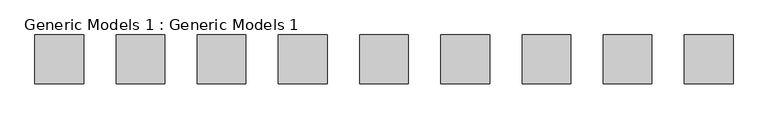
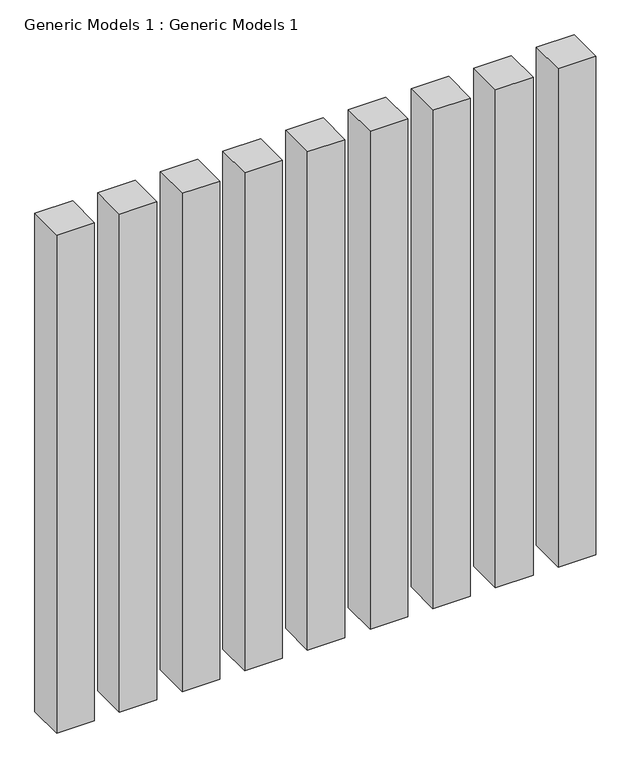
"""IFC4 building model written with IfcOpenShell, lengths in millimetres: proxy geometry, Generic Models 1 : Generic Models 1."""

from ifc_helpers import new_model, si_unit, origin, origin_with_axes, place, context, project, spatial, polyline, outline, extrude, source, transform, mapped, element, save


def generic_models_1_generic_models_1_04f99ef1(model_context):
    return source(origin(), model_context, "Body", "SweptSolid", [
        extrude(outline(polyline([(23542.6546318, -2836.165108), (23314.0546318, -2836.165108), (23314.0546318, -2607.565108), (23542.6546318, -2607.565108), (23542.6546318, -2836.165108)])), origin_with_axes(), (0.0, 0.0, 1.0), 3200.4),
        extrude(outline(polyline([(23923.6546318, -2836.165108), (23695.0546318, -2836.165108), (23695.0546318, -2607.565108), (23923.6546318, -2607.565108), (23923.6546318, -2836.165108)])), origin_with_axes(), (0.0, 0.0, 1.0), 3200.4),
        extrude(outline(polyline([(24304.6546318, -2836.165108), (24076.0546318, -2836.165108), (24076.0546318, -2607.565108), (24304.6546318, -2607.565108), (24304.6546318, -2836.165108)])), origin_with_axes(), (0.0, 0.0, 1.0), 3200.4),
        extrude(outline(polyline([(24685.6546318, -2836.165108), (24457.0546318, -2836.165108), (24457.0546318, -2607.565108), (24685.6546318, -2607.565108), (24685.6546318, -2836.165108)])), origin_with_axes(), (0.0, 0.0, 1.0), 3200.4),
        extrude(outline(polyline([(25066.6546318, -2836.165108), (24838.0546318, -2836.165108), (24838.0546318, -2607.565108), (25066.6546318, -2607.565108), (25066.6546318, -2836.165108)])), origin_with_axes(), (0.0, 0.0, 1.0), 3200.4),
        extrude(outline(polyline([(25447.6546318, -2836.165108), (25219.0546318, -2836.165108), (25219.0546318, -2607.565108), (25447.6546318, -2607.565108), (25447.6546318, -2836.165108)])), origin_with_axes(), (0.0, 0.0, 1.0), 3200.4),
        extrude(outline(polyline([(25828.6546318, -2836.165108), (25600.0546318, -2836.165108), (25600.0546318, -2607.565108), (25828.6546318, -2607.565108), (25828.6546318, -2836.165108)])), origin_with_axes(), (0.0, 0.0, 1.0), 3200.4),
        extrude(outline(polyline([(26209.6546318, -2836.165108), (25981.0546318, -2836.165108), (25981.0546318, -2607.565108), (26209.6546318, -2607.565108), (26209.6546318, -2836.165108)])), origin_with_axes(), (0.0, 0.0, 1.0), 3200.4),
        extrude(outline(polyline([(26590.6546318, -2836.165108), (26362.0546318, -2836.165108), (26362.0546318, -2607.565108), (26590.6546318, -2607.565108), (26590.6546318, -2836.165108)])), origin_with_axes(), (0.0, 0.0, 1.0), 3200.4),
    ])


if __name__ == "__main__":
    model = new_model("IFC4")
    model_context = context("Model", 3, world=origin())
    ifc_project = project(units=[si_unit("LENGTHUNIT", "METRE", prefix="MILLI")], contexts=[model_context])
    site = spatial("IfcSite", under=ifc_project)
    building = spatial("IfcBuilding", under=site)
    placement = place(None, origin())
    generic_models_1_generic_models_1_shape = generic_models_1_generic_models_1_04f99ef1(model_context)
    element("IfcBuildingElementProxy", 1, Name="Generic Models 1 : Generic Models 1", ObjectType="Generic Models 1 : Generic Models 1", at=placement, inside=building, context=model_context, shape_type="MappedRepresentation", body=[
        mapped(generic_models_1_generic_models_1_shape, transform((0.0, 0.0, 0.0), x_axis=(1.0, 0.0, 0.0), y_axis=(0.0, 1.0, 0.0), z_axis=(0.0, 0.0, 1.0))),
    ])
    save(model, "model.ifc")

# Revit data of these elements
# Element 1 (IfcBuildingElementProxy, "Generic Models 1 : Generic Models 1")
#   Materials on its faces: "0 olive green"
# Materials
#   "0 olive green": class "Generic", colour RGB 120 120 120, transparency 0, Cost = 0
